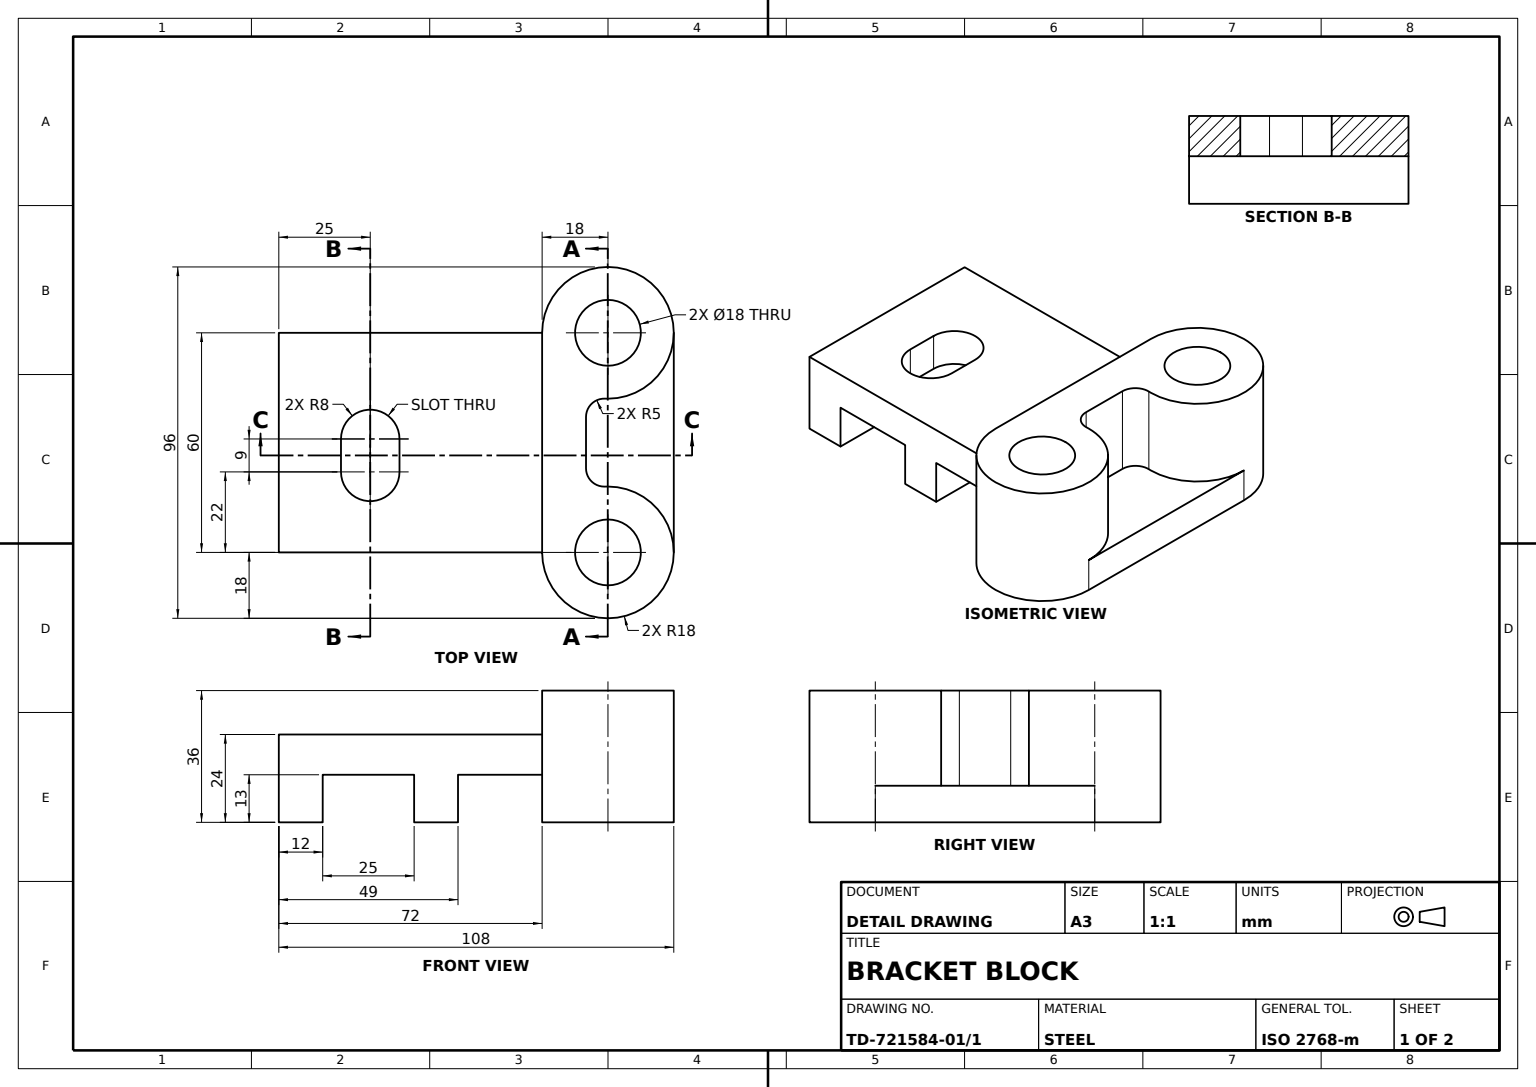
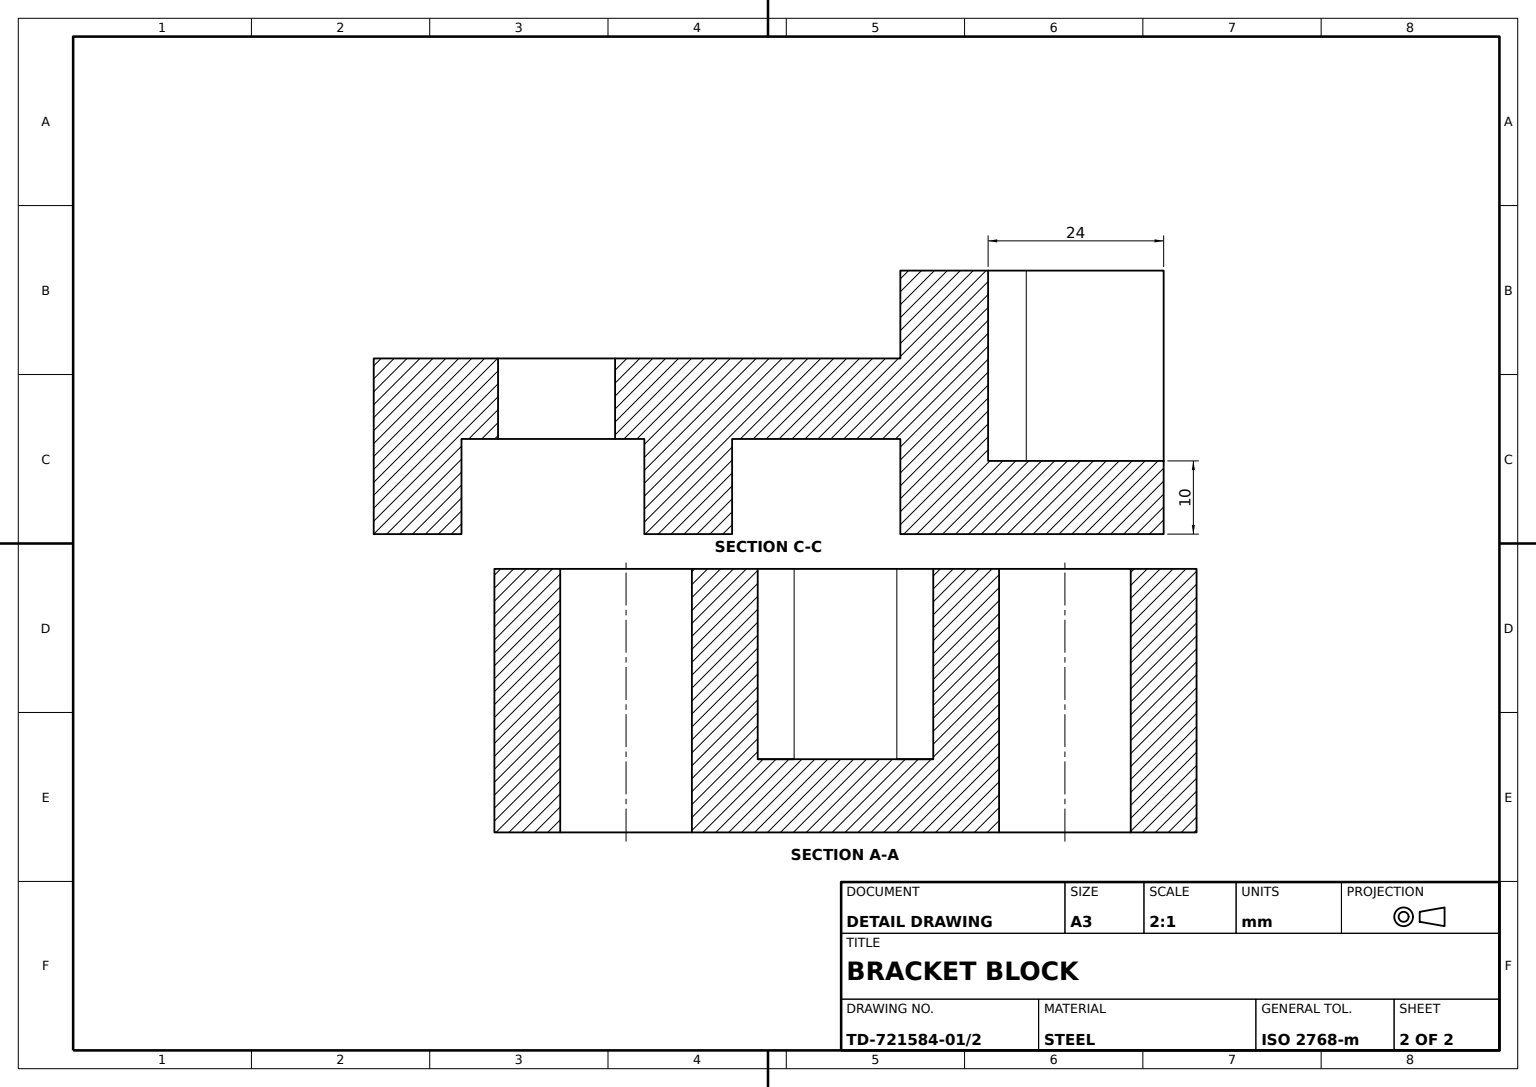
from build123d import *

# Parameters (mm, degrees)
BASE_BLOCK_DEPTH          = 60
TWIN_LUG_PROFILE_SKETCH_R = 9
TWIN_LUGS_DEPTH           = 36
LUG_START                 = 10
LUG_WEB_DEPTH             = 10
MOUNTING_SLOT_9MM_DEPTH   = 136.366170072


with BuildPart() as part:
    # Base Block Profile Sketch → Base Block (new body)
    with BuildSketch(Plane.XY):
        Polygon((0, 0), (12, 0), (12, 13), (37, 13), (37, 0), (49, 0), (49, 13), (72, 13), (72, 24), (0, 24), align=None)
    extrude(amount=BASE_BLOCK_DEPTH)

    # Twin Lug Profile Sketch → Twin Lugs (add)
    with BuildSketch(Plane(origin=(0, 36, 0), x_dir=(1, 0, 0), z_dir=(0, 1, 0))):
        with BuildLine():
            Line((72, 0), (72, -60))
            ThreePointArc((72, -60), (103.001672133, -72.448153347), (89.217391304, -42.01702128))
            ThreePointArc((89.217391304, -42.01702128), (85.542179626, -40.633325006), (84, -37.021749414))
            Line((84, -37.021749414), (84, -22.978250586))
            ThreePointArc((84, -22.978250586), (85.542179626, -19.366674994), (89.217391304, -17.98297872))
            ThreePointArc((89.217391304, -17.98297872), (103.001672133, 12.448153347), (72, 0))
        make_face()
        with Locations(Location((90, 0, 0), (0, 0, 270))):
            Circle(TWIN_LUG_PROFILE_SKETCH_R, mode=Mode.SUBTRACT)
        with Locations(Location((90, -60, 0), (0, 0, 270))):
            Circle(TWIN_LUG_PROFILE_SKETCH_R, mode=Mode.SUBTRACT)
    extrude(amount=-TWIN_LUGS_DEPTH)

    # Lug Web Profile Sketch → Lug Web (add)
    with BuildSketch(Plane(origin=(0, 0, 0), x_dir=(1, 0, 0), z_dir=(0, 1, 0)).offset(LUG_START)):
        with BuildLine():
            Line((108, -60), (108, 0))
            ThreePointArc((108, 0), (102.448153347, -13.001672133), (89.217391304, -17.98297872))
            ThreePointArc((89.217391304, -17.98297872), (85.542179626, -19.366674994), (84, -22.978250586))
            Line((84, -22.978250586), (84, -37.021749414))
            ThreePointArc((84, -37.021749414), (85.241609163, -40.399518098), (88.429875668, -42.068611053))
            ThreePointArc((88.429875668, -42.068611053), (89.214188653, -42.017160944), (90, -42))
            ThreePointArc((90, -42), (102.727922061, -47.272077939), (108, -60))
        make_face()
    extrude(amount=-LUG_WEB_DEPTH)

    # Mounting Slot Sketch → Mounting Slot 9mm (cut, through all)
    with BuildSketch(Plane(origin=(0, 24, 0), x_dir=(1, 0, 0), z_dir=(0, 1, 0))):
        with BuildLine():
            Line((33, -29), (33, -38))
            ThreePointArc((33, -38), (25, -46), (17, -38))
            Line((17, -38), (17, -29))
            ThreePointArc((17, -29), (25, -21), (33, -29))
        make_face()
    extrude(amount=-MOUNTING_SLOT_9MM_DEPTH, mode=Mode.SUBTRACT)


solid = part.part
